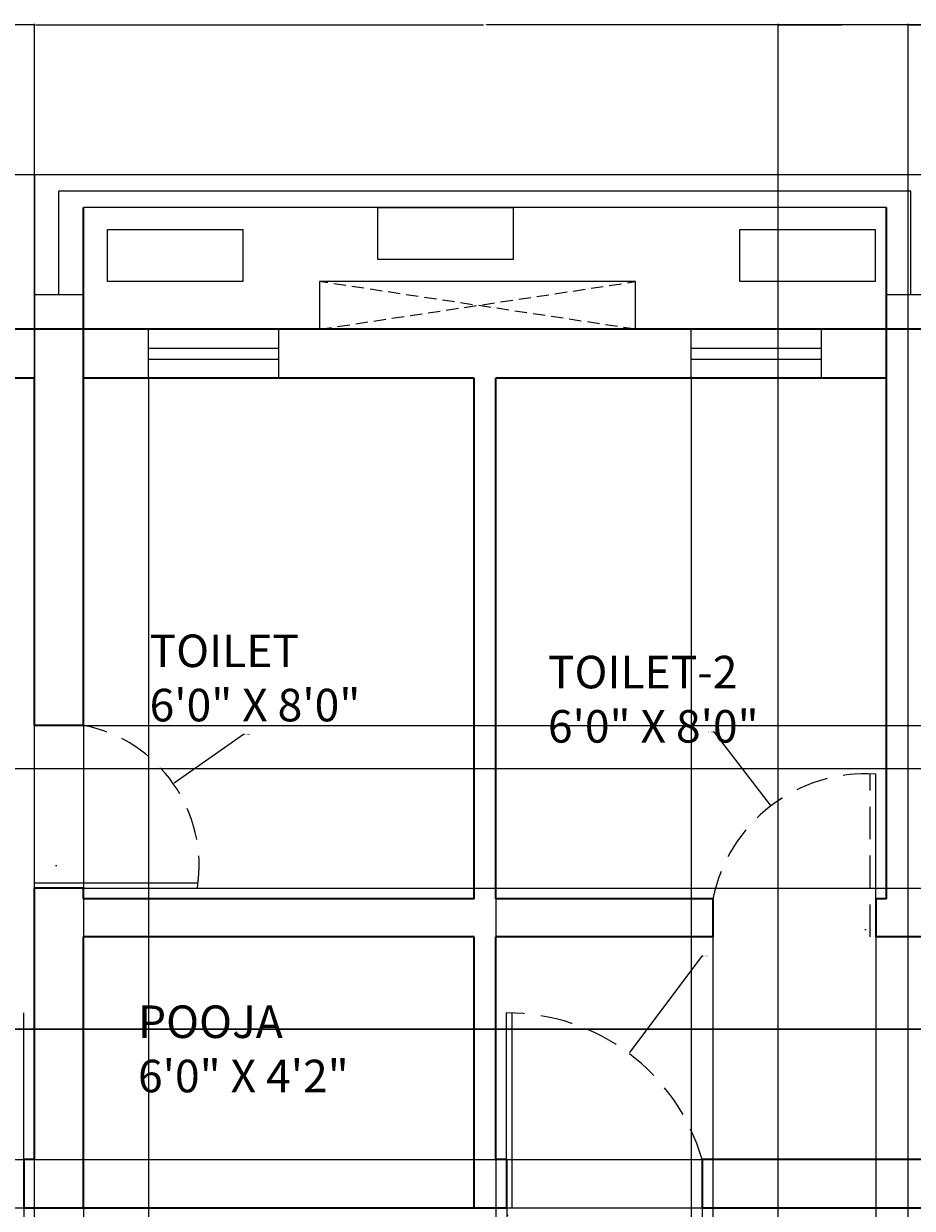
# Model space of a CAD drawing. Units: inches. Extents: x 6662 to 7211, y 5077 to 5683.
# Tile 8 of 9: x 6868 to 7032, y 5465 to 5683. Entities that reach past the tile are written whole.
import ezdxf

# ---------------------------------------------------------------- set-up
doc = ezdxf.new("R2010")
doc.units = ezdxf.units.IN
doc.header["$LTSCALE"] = 3
doc.header["$MEASUREMENT"] = 0
doc.linetypes.add('HIDDEN', pattern=[0.375, 0.25, -0.125])
for name, color, linetype, lineweight in [('A-ANNO-DIMS', 2, 'Continuous', 18), ('A-AREA-IDEN', 7, 'Continuous', 18), ('A-DOOR', 4, 'Continuous', 25), ('A-DOOR-HIDN', 4, 'HIDDEN', 13), ('A-FLOR-CASE-PATT', 241, 'Continuous', 13), ('A-FLOR-PROJ', 7, 'Continuous', 18), ('A-FLOR-PROJ-HIDN', 7, 'HIDDEN', 13), ('A-GLAZ', 4, 'Continuous', 18), ('A-WALL', 7, 'Continuous', 35)]:
    doc.layers.add(name, color=color, linetype=linetype, lineweight=lineweight)
doc.styles.get("Standard").update_dxf_attribs({"font": 'arial.ttf'})
doc.dimstyles.get("Standard").update_dxf_attribs({"dimtxt": 0.18, "dimasz": 0.18, "dimexe": 0.18, "dimexo": 0.0625, "dimgap": 0.09, "dimtad": 0, "dimtih": 1, "dimtoh": 1, "dimdec": 4, "dimzin": 0, "dimdsep": 46, "dimtxsty": 'Standard', "dimcen": 0.09, "dimadec": 0, "dimazin": 0, "dimtfac": 1, "dimtdec": 4, "dimtofl": 0, "dimtmove": 0, "dimatfit": 3, "dimfxl": 1, "dimtolj": 1, "dimtzin": 0, "dimarcsym": 0})

# ---------------------------------------------------------------- blocks, each defined once
blk = doc.blocks.new('WIN-VENT-24IN')
for p, q in [((0, 0), (0, 9)), ((24, 0), (24, 9)), ((0, 5.5), (24, 5.5)), ((0, 3.5), (24, 3.5))]:
    blk.add_line(p, q)
blk = doc.blocks.new('*D41')
at = {"layer": 'A-ANNO-DIMS', "color": 0, "lineweight": -2, "ltscale": 3, "transparency": 16777216}
for p, q in [((7035.92, 5655.02), (7210.74, 5655.02)), ((7210.56, 5654.84), (7210.56, 5379.99)), ((7210.56, 5104.78), (7210.56, 5379.63)), ((7010.92, 5104.6), (7210.74, 5104.6))]:
    blk.add_line(p, q, dxfattribs=at)
at = {"layer": 'A-ANNO-DIMS', "color": 0, "ltscale": 3, "transparency": 16777216}
for points in [[(7210.53, 5654.84), (7210.59, 5654.84), (7210.56, 5655.02)], [(7210.53, 5104.78), (7210.59, 5104.78), (7210.56, 5104.6)]]:
    blk.add_solid(points, dxfattribs=at)
at = {"layer": 'Defpoints', "color": 0, "ltscale": 3, "transparency": 16777216}
for p in [(7035.86, 5655.02), (7210.56, 5655.02), (7010.86, 5104.6)]:
    blk.add_point(p, dxfattribs=at)
at = {"layer": 'A-ANNO-DIMS', "color": 0, "ltscale": 3, "transparency": 16777216, "insert": (7210.56, 5379.81), "char_height": 0.18, "attachment_point": 5}
blk.add_mtext('\\A1;550.4', dxfattribs=at)
blk = doc.blocks.new('*D45')
at = {"layer": 'A-ANNO-DIMS', "color": 0, "lineweight": -2, "ltscale": 3, "transparency": 16777216}
for p, q in [((6845.86, 5626.66), (6845.86, 5682.9)), ((6846.04, 5682.72), (6857.64, 5682.72)), ((6869.68, 5682.72), (6858.08, 5682.72)), ((6869.86, 5655.08), (6869.86, 5682.9))]:
    blk.add_line(p, q, dxfattribs=at)
at = {"layer": 'A-ANNO-DIMS', "color": 0, "ltscale": 3, "transparency": 16777216}
for points in [[(6846.04, 5682.75), (6846.04, 5682.69), (6845.86, 5682.72)], [(6869.68, 5682.75), (6869.68, 5682.69), (6869.86, 5682.72)]]:
    blk.add_solid(points, dxfattribs=at)
at = {"layer": 'Defpoints', "color": 0, "ltscale": 3, "transparency": 16777216}
for p in [(6869.86, 5682.72), (6869.86, 5655.02), (6845.86, 5626.6)]:
    blk.add_point(p, dxfattribs=at)
at = {"layer": 'A-ANNO-DIMS', "color": 0, "ltscale": 3, "transparency": 16777216, "insert": (6857.86, 5682.72), "char_height": 0.18, "attachment_point": 5}
blk.add_mtext('\\A1;24', dxfattribs=at)
blk = doc.blocks.new('*D46')
at = {"layer": 'A-ANNO-DIMS', "color": 0, "lineweight": -2, "ltscale": 3, "transparency": 16777216}
for p, q in [((6869.86, 5655.08), (6869.86, 5682.9)), ((6870.04, 5682.72), (6952.58, 5682.72)), ((7035.68, 5682.72), (6953.14, 5682.72)), ((7035.86, 5655.08), (7035.86, 5682.9))]:
    blk.add_line(p, q, dxfattribs=at)
at = {"layer": 'A-ANNO-DIMS', "color": 0, "ltscale": 3, "transparency": 16777216}
for points in [[(6870.04, 5682.75), (6870.04, 5682.69), (6869.86, 5682.72)], [(7035.68, 5682.75), (7035.68, 5682.69), (7035.86, 5682.72)]]:
    blk.add_solid(points, dxfattribs=at)
at = {"layer": 'Defpoints', "color": 0, "ltscale": 3, "transparency": 16777216}
for p in [(7035.86, 5682.72), (6869.86, 5655.02), (7035.86, 5655.02)]:
    blk.add_point(p, dxfattribs=at)
at = {"layer": 'A-ANNO-DIMS', "color": 0, "ltscale": 3, "transparency": 16777216, "insert": (6952.86, 5682.72), "char_height": 0.18, "attachment_point": 5}
blk.add_mtext('\\A1;166', dxfattribs=at)
blk = doc.blocks.new('*D50')
at = {"layer": 'A-ANNO-DIMS', "color": 0, "lineweight": -2, "ltscale": 3, "transparency": 16777216}
for p, q in [((6869.8, 5655.02), (6661.98, 5655.02)), ((6662.16, 5654.84), (6662.16, 5640.99)), ((6662.16, 5626.78), (6662.16, 5640.63)), ((6716.8, 5626.6), (6661.98, 5626.6))]:
    blk.add_line(p, q, dxfattribs=at)
at = {"layer": 'A-ANNO-DIMS', "color": 0, "ltscale": 3, "transparency": 16777216}
for points in [[(6662.13, 5654.84), (6662.19, 5654.84), (6662.16, 5655.02)], [(6662.13, 5626.78), (6662.19, 5626.78), (6662.16, 5626.6)]]:
    blk.add_solid(points, dxfattribs=at)
at = {"layer": 'Defpoints', "color": 0, "ltscale": 3, "transparency": 16777216}
for p in [(6662.16, 5655.02), (6869.86, 5655.02), (6716.86, 5626.6)]:
    blk.add_point(p, dxfattribs=at)
at = {"layer": 'A-ANNO-DIMS', "color": 0, "ltscale": 3, "transparency": 16777216, "insert": (6662.16, 5640.81), "char_height": 0.18, "attachment_point": 5}
blk.add_mtext('\\A1;28.423', dxfattribs=at)
blk = doc.blocks.new('*D64')
at = {"layer": 'A-ANNO-DIMS', "color": 0, "lineweight": -2, "ltscale": 3, "transparency": 16777216}
for p, q in [((6833.86, 5332.16), (6833.86, 5682.9)), ((6834.04, 5682.72), (6851.64, 5682.72)), ((6869.68, 5682.72), (6852.08, 5682.72)), ((6869.86, 5332.16), (6869.86, 5682.9))]:
    blk.add_line(p, q, dxfattribs=at)
at = {"layer": 'A-ANNO-DIMS', "color": 0, "ltscale": 3, "transparency": 16777216}
for points in [[(6834.04, 5682.75), (6834.04, 5682.69), (6833.86, 5682.72)], [(6869.68, 5682.75), (6869.68, 5682.69), (6869.86, 5682.72)]]:
    blk.add_solid(points, dxfattribs=at)
at = {"layer": 'Defpoints', "color": 0, "ltscale": 3, "transparency": 16777216}
for p in [(6869.86, 5682.72), (6833.86, 5332.1), (6869.86, 5332.1)]:
    blk.add_point(p, dxfattribs=at)
at = {"layer": 'A-ANNO-DIMS', "color": 0, "ltscale": 3, "transparency": 16777216, "insert": (6851.86, 5682.72), "char_height": 0.18, "attachment_point": 5}
blk.add_mtext('\\A1;36', dxfattribs=at)
blk = doc.blocks.new('*D65')
at = {"layer": 'A-ANNO-DIMS', "color": 0, "lineweight": -2, "ltscale": 3, "transparency": 16777216}
for p, q in [((6831.86, 5464.54), (6831.86, 5076.72)), ((6867.86, 5464.54), (6867.86, 5076.72)), ((6832.04, 5076.9), (6849.64, 5076.9)), ((6867.68, 5076.9), (6850.08, 5076.9))]:
    blk.add_line(p, q, dxfattribs=at)
at = {"layer": 'A-ANNO-DIMS', "color": 0, "ltscale": 3, "transparency": 16777216}
for points in [[(6832.04, 5076.93), (6832.04, 5076.87), (6831.86, 5076.9)], [(6867.68, 5076.93), (6867.68, 5076.87), (6867.86, 5076.9)]]:
    blk.add_solid(points, dxfattribs=at)
at = {"layer": 'Defpoints', "color": 0, "ltscale": 3, "transparency": 16777216}
for p in [(6831.86, 5464.6), (6867.86, 5464.6), (6867.86, 5076.9)]:
    blk.add_point(p, dxfattribs=at)
at = {"layer": 'A-ANNO-DIMS', "color": 0, "ltscale": 3, "transparency": 16777216, "insert": (6849.86, 5076.9), "char_height": 0.18, "attachment_point": 5}
blk.add_mtext('\\A1;36', dxfattribs=at)
blk = doc.blocks.new('*D66')
at = {"layer": 'A-ANNO-DIMS', "color": 0, "lineweight": -2, "ltscale": 3, "transparency": 16777216}
for p, q in [((6956.86, 5464.54), (6956.86, 5076.72)), ((6992.86, 5464.54), (6992.86, 5076.72)), ((6957.04, 5076.9), (6974.64, 5076.9)), ((6992.68, 5076.9), (6975.08, 5076.9))]:
    blk.add_line(p, q, dxfattribs=at)
at = {"layer": 'A-ANNO-DIMS', "color": 0, "ltscale": 3, "transparency": 16777216}
for points in [[(6957.04, 5076.93), (6957.04, 5076.87), (6956.86, 5076.9)], [(6992.68, 5076.93), (6992.68, 5076.87), (6992.86, 5076.9)]]:
    blk.add_solid(points, dxfattribs=at)
at = {"layer": 'Defpoints', "color": 0, "ltscale": 3, "transparency": 16777216}
for p in [(6956.86, 5464.6), (6992.86, 5464.6), (6992.86, 5076.9)]:
    blk.add_point(p, dxfattribs=at)
at = {"layer": 'A-ANNO-DIMS', "color": 0, "ltscale": 3, "transparency": 16777216, "insert": (6974.86, 5076.9), "char_height": 0.18, "attachment_point": 5}
blk.add_mtext('\\A1;36', dxfattribs=at)
blk = doc.blocks.new('*D67')
at = {"layer": 'A-ANNO-DIMS', "color": 0, "lineweight": -2, "ltscale": 3, "transparency": 16777216}
for p, q in [((6994.86, 5514.54), (6994.86, 5076.72)), ((7024.86, 5514.54), (7024.86, 5076.72)), ((6995.04, 5076.9), (7009.64, 5076.9)), ((7024.68, 5076.9), (7010.08, 5076.9))]:
    blk.add_line(p, q, dxfattribs=at)
at = {"layer": 'A-ANNO-DIMS', "color": 0, "ltscale": 3, "transparency": 16777216}
for points in [[(6995.04, 5076.93), (6995.04, 5076.87), (6994.86, 5076.9)], [(7024.68, 5076.93), (7024.68, 5076.87), (7024.86, 5076.9)]]:
    blk.add_solid(points, dxfattribs=at)
at = {"layer": 'Defpoints', "color": 0, "ltscale": 3, "transparency": 16777216}
for p in [(6994.86, 5514.6), (7024.86, 5514.6), (7024.86, 5076.9)]:
    blk.add_point(p, dxfattribs=at)
at = {"layer": 'A-ANNO-DIMS', "color": 0, "ltscale": 3, "transparency": 16777216, "insert": (7009.86, 5076.9), "char_height": 0.18, "attachment_point": 5}
blk.add_mtext('\\A1;30', dxfattribs=at)
blk = doc.blocks.new('*D68')
at = {"layer": 'A-ANNO-DIMS', "color": 0, "lineweight": -2, "ltscale": 3, "transparency": 16777216}
for p, q in [((6878.92, 5553.6), (7210.74, 5553.6)), ((7210.56, 5553.42), (7210.56, 5538.78)), ((7210.56, 5523.78), (7210.56, 5538.42)), ((6878.92, 5523.6), (7210.74, 5523.6))]:
    blk.add_line(p, q, dxfattribs=at)
at = {"layer": 'A-ANNO-DIMS', "color": 0, "ltscale": 3, "transparency": 16777216}
for points in [[(7210.53, 5553.42), (7210.59, 5553.42), (7210.56, 5553.6)], [(7210.53, 5523.78), (7210.59, 5523.78), (7210.56, 5523.6)]]:
    blk.add_solid(points, dxfattribs=at)
at = {"layer": 'Defpoints', "color": 0, "ltscale": 3, "transparency": 16777216}
for p in [(6878.86, 5553.6), (7210.56, 5553.6), (6878.86, 5523.6)]:
    blk.add_point(p, dxfattribs=at)
at = {"layer": 'A-ANNO-DIMS', "color": 0, "ltscale": 3, "transparency": 16777216, "insert": (7210.56, 5538.6), "char_height": 0.18, "attachment_point": 5}
blk.add_mtext('\\A1;30', dxfattribs=at)
blk = doc.blocks.new('*D71')
at = {"layer": 'A-ANNO-DIMS', "color": 0, "lineweight": -2, "ltscale": 3, "transparency": 16777216}
for p, q in [((6878.86, 5617.54), (6878.86, 5076.72)), ((6890.86, 5617.54), (6890.86, 5076.72)), ((6879.04, 5076.9), (6884.65, 5076.9)), ((6890.68, 5076.9), (6885.07, 5076.9))]:
    blk.add_line(p, q, dxfattribs=at)
at = {"layer": 'A-ANNO-DIMS', "color": 0, "ltscale": 3, "transparency": 16777216}
for points in [[(6879.04, 5076.93), (6879.04, 5076.87), (6878.86, 5076.9)], [(6890.68, 5076.93), (6890.68, 5076.87), (6890.86, 5076.9)]]:
    blk.add_solid(points, dxfattribs=at)
at = {"layer": 'Defpoints', "color": 0, "ltscale": 3, "transparency": 16777216}
for p in [(6878.86, 5617.6), (6890.86, 5617.6), (6878.86, 5076.9)]:
    blk.add_point(p, dxfattribs=at)
at = {"layer": 'A-ANNO-DIMS', "color": 0, "ltscale": 3, "transparency": 16777216, "insert": (6884.86, 5076.9), "char_height": 0.18, "attachment_point": 5}
blk.add_mtext('\\A1;12', dxfattribs=at)
blk = doc.blocks.new('*D72')
at = {"layer": 'A-ANNO-DIMS', "color": 0, "lineweight": -2, "ltscale": 3, "transparency": 16777216}
for p, q in [((6954.86, 5617.54), (6954.86, 5076.72)), ((6990.86, 5617.54), (6990.86, 5076.72)), ((6955.04, 5076.9), (6972.64, 5076.9)), ((6990.68, 5076.9), (6973.08, 5076.9))]:
    blk.add_line(p, q, dxfattribs=at)
at = {"layer": 'A-ANNO-DIMS', "color": 0, "ltscale": 3, "transparency": 16777216}
for points in [[(6955.04, 5076.93), (6955.04, 5076.87), (6954.86, 5076.9)], [(6990.68, 5076.93), (6990.68, 5076.87), (6990.86, 5076.9)]]:
    blk.add_solid(points, dxfattribs=at)
at = {"layer": 'Defpoints', "color": 0, "ltscale": 3, "transparency": 16777216}
for p in [(6954.86, 5617.6), (6990.86, 5617.6), (6990.86, 5076.9)]:
    blk.add_point(p, dxfattribs=at)
at = {"layer": 'A-ANNO-DIMS', "color": 0, "ltscale": 3, "transparency": 16777216, "insert": (6972.86, 5076.9), "char_height": 0.18, "attachment_point": 5}
blk.add_mtext('\\A1;36', dxfattribs=at)
blk = doc.blocks.new('*D74')
at = {"layer": 'A-ANNO-DIMS', "color": 0, "lineweight": -2, "ltscale": 3, "transparency": 16777216}
for p, q in [((7006.86, 5179.16), (7006.86, 5682.9)), ((7007.04, 5682.72), (7018.64, 5682.72)), ((7030.68, 5682.72), (7019.08, 5682.72)), ((7030.86, 5179.16), (7030.86, 5682.9))]:
    blk.add_line(p, q, dxfattribs=at)
at = {"layer": 'A-ANNO-DIMS', "color": 0, "ltscale": 3, "transparency": 16777216}
for points in [[(7007.04, 5682.75), (7007.04, 5682.69), (7006.86, 5682.72)], [(7030.68, 5682.75), (7030.68, 5682.69), (7030.86, 5682.72)]]:
    blk.add_solid(points, dxfattribs=at)
at = {"layer": 'Defpoints', "color": 0, "ltscale": 3, "transparency": 16777216}
for p in [(7030.86, 5682.72), (7006.86, 5179.1), (7030.86, 5179.1)]:
    blk.add_point(p, dxfattribs=at)
at = {"layer": 'A-ANNO-DIMS', "color": 0, "ltscale": 3, "transparency": 16777216, "insert": (7018.86, 5682.72), "char_height": 0.18, "attachment_point": 5}
blk.add_mtext('\\A1;24', dxfattribs=at)
blk = doc.blocks.new('*D75')
at = {"layer": 'A-ANNO-DIMS', "color": 0, "lineweight": -2, "ltscale": 3, "transparency": 16777216}
for p, q in [((7030.86, 5179.16), (7030.86, 5682.9)), ((7031.04, 5682.72), (7054.64, 5682.72)), ((7078.68, 5682.72), (7055.08, 5682.72)), ((7078.86, 5179.16), (7078.86, 5682.9))]:
    blk.add_line(p, q, dxfattribs=at)
at = {"layer": 'A-ANNO-DIMS', "color": 0, "ltscale": 3, "transparency": 16777216}
for points in [[(7031.04, 5682.75), (7031.04, 5682.69), (7030.86, 5682.72)], [(7078.68, 5682.75), (7078.68, 5682.69), (7078.86, 5682.72)]]:
    blk.add_solid(points, dxfattribs=at)
at = {"layer": 'Defpoints', "color": 0, "ltscale": 3, "transparency": 16777216}
for p in [(7078.86, 5682.72), (7030.86, 5179.1), (7078.86, 5179.1)]:
    blk.add_point(p, dxfattribs=at)
at = {"layer": 'A-ANNO-DIMS', "color": 0, "ltscale": 3, "transparency": 16777216, "insert": (7054.86, 5682.72), "char_height": 0.18, "attachment_point": 5}
blk.add_mtext('\\A1;48', dxfattribs=at)
blk = doc.blocks.new('*D76')
at = {"layer": 'A-ANNO-DIMS', "color": 0, "lineweight": -2, "ltscale": 3, "transparency": 16777216}
for p, q in [((7167.8, 5464.6), (6661.98, 5464.6)), ((6662.16, 5464.42), (6662.16, 5449.65)), ((6662.16, 5434.53), (6662.16, 5449.29)), ((7167.8, 5434.35), (6661.98, 5434.35))]:
    blk.add_line(p, q, dxfattribs=at)
at = {"layer": 'A-ANNO-DIMS', "color": 0, "ltscale": 3, "transparency": 16777216}
for points in [[(6662.13, 5464.42), (6662.19, 5464.42), (6662.16, 5464.6)], [(6662.13, 5434.53), (6662.19, 5434.53), (6662.16, 5434.35)]]:
    blk.add_solid(points, dxfattribs=at)
at = {"layer": 'Defpoints', "color": 0, "ltscale": 3, "transparency": 16777216}
for p in [(7167.86, 5464.6), (6662.16, 5434.35), (7167.86, 5434.35)]:
    blk.add_point(p, dxfattribs=at)
at = {"layer": 'A-ANNO-DIMS', "color": 0, "ltscale": 3, "transparency": 16777216, "insert": (6662.16, 5449.47), "char_height": 0.18, "attachment_point": 5}
blk.add_mtext('\\A1;30.25', dxfattribs=at)
blk = doc.blocks.new('*D80')
at = {"layer": 'A-ANNO-DIMS', "color": 0, "lineweight": -2, "ltscale": 3, "transparency": 16777216}
for p, q in [((6825.96, 5497.6), (7210.74, 5497.6)), ((7210.56, 5497.42), (7210.56, 5485.78)), ((7210.56, 5473.78), (7210.56, 5485.42)), ((6825.96, 5473.6), (7210.74, 5473.6))]:
    blk.add_line(p, q, dxfattribs=at)
at = {"layer": 'A-ANNO-DIMS', "color": 0, "ltscale": 3, "transparency": 16777216}
for points in [[(7210.53, 5497.42), (7210.59, 5497.42), (7210.56, 5497.6)], [(7210.53, 5473.78), (7210.59, 5473.78), (7210.56, 5473.6)]]:
    blk.add_solid(points, dxfattribs=at)
at = {"layer": 'Defpoints', "color": 0, "ltscale": 3, "transparency": 16777216}
for p in [(6825.9, 5497.6), (7210.56, 5497.6), (6825.9, 5473.6)]:
    blk.add_point(p, dxfattribs=at)
at = {"layer": 'A-ANNO-DIMS', "color": 0, "ltscale": 3, "transparency": 16777216, "insert": (7210.56, 5485.6), "char_height": 0.18, "attachment_point": 5}
blk.add_mtext('\\A1;24', dxfattribs=at)
blk = doc.blocks.new('*D82')
at = {"layer": 'A-ANNO-DIMS', "color": 0, "lineweight": -2, "ltscale": 3, "transparency": 16777216}
for p, q in [((7167.8, 5545.6), (6661.98, 5545.6)), ((6662.16, 5545.42), (6662.16, 5521.78)), ((6662.16, 5497.78), (6662.16, 5521.42)), ((7167.8, 5497.6), (6661.98, 5497.6))]:
    blk.add_line(p, q, dxfattribs=at)
at = {"layer": 'A-ANNO-DIMS', "color": 0, "ltscale": 3, "transparency": 16777216}
for points in [[(6662.13, 5545.42), (6662.19, 5545.42), (6662.16, 5545.6)], [(6662.13, 5497.78), (6662.19, 5497.78), (6662.16, 5497.6)]]:
    blk.add_solid(points, dxfattribs=at)
at = {"layer": 'Defpoints', "color": 0, "ltscale": 3, "transparency": 16777216}
for p in [(6662.16, 5545.6), (7167.86, 5545.6), (7167.86, 5497.6)]:
    blk.add_point(p, dxfattribs=at)
at = {"layer": 'A-ANNO-DIMS', "color": 0, "ltscale": 3, "transparency": 16777216, "insert": (6662.16, 5521.6), "char_height": 0.18, "attachment_point": 5}
blk.add_mtext('\\A1;48', dxfattribs=at)
blk = doc.blocks.new('*D88')
at = {"layer": 'A-ANNO-DIMS', "color": 0, "lineweight": -2, "ltscale": 3, "transparency": 16777216}
for p, q in [((6992.81, 5511.04), (6979.5, 5493.29)), ((6992.99, 5511.04), (6992.81, 5511.04)), ((6956.93, 5463.31), (6957.11, 5463.31)), ((6957.02, 5463.22), (6957.02, 5463.4))]:
    blk.add_line(p, q, dxfattribs=at)
at = {"layer": 'A-ANNO-DIMS', "color": 0, "ltscale": 3, "transparency": 16777216}
blk.add_solid([(6979.47, 5493.3), (6979.52, 5493.27), (6979.39, 5493.14)], dxfattribs=at)
at = {"layer": 'Defpoints', "color": 0, "ltscale": 3, "transparency": 16777216}
for p in [(6979.39, 5493.14), (6957.02, 5463.31)]:
    blk.add_point(p, dxfattribs=at)
at = {"layer": 'A-ANNO-DIMS', "color": 0, "ltscale": 3, "transparency": 16777216, "insert": (6993.54, 5511.04), "char_height": 0.18, "attachment_point": 5}
blk.add_mtext('\\A1;R37.285', dxfattribs=at)
blk = doc.blocks.new('*D93')
at = {"layer": 'A-ANNO-DIMS', "color": 0, "lineweight": -2, "ltscale": 3, "transparency": 16777216}
for p, q in [((6994.88, 5552.4), (6995.06, 5552.4)), ((6995.06, 5552.4), (7005.42, 5538.88)), ((7022.9, 5515.97), (7023.08, 5515.97)), ((7022.99, 5515.88), (7022.99, 5516.06))]:
    blk.add_line(p, q, dxfattribs=at)
at = {"layer": 'A-ANNO-DIMS', "color": 0, "ltscale": 3, "transparency": 16777216}
blk.add_solid([(7005.45, 5538.9), (7005.4, 5538.86), (7005.53, 5538.74)], dxfattribs=at)
at = {"layer": 'Defpoints', "color": 0, "ltscale": 3, "transparency": 16777216}
for p in [(7005.53, 5538.74), (7022.99, 5515.97)]:
    blk.add_point(p, dxfattribs=at)
at = {"layer": 'A-ANNO-DIMS', "color": 0, "ltscale": 3, "transparency": 16777216, "insert": (6994.4, 5552.4), "char_height": 0.18, "attachment_point": 5}
blk.add_mtext('\\A1;R28.69', dxfattribs=at)
blk = doc.blocks.new('*D95')
at = {"layer": 'A-ANNO-DIMS', "color": 0, "lineweight": -2, "ltscale": 3, "transparency": 16777216}
for p, q in [((6908.37, 5551.9), (6895.58, 5542.95)), ((6908.55, 5551.9), (6908.37, 5551.9)), ((6873.78, 5527.76), (6873.96, 5527.76)), ((6873.87, 5527.67), (6873.87, 5527.85))]:
    blk.add_line(p, q, dxfattribs=at)
at = {"layer": 'A-ANNO-DIMS', "color": 0, "ltscale": 3, "transparency": 16777216}
blk.add_solid([(6895.56, 5542.98), (6895.6, 5542.93), (6895.43, 5542.85)], dxfattribs=at)
at = {"layer": 'Defpoints', "color": 0, "ltscale": 3, "transparency": 16777216}
for p in [(6895.43, 5542.85), (6873.87, 5527.76)]:
    blk.add_point(p, dxfattribs=at)
at = {"layer": 'A-ANNO-DIMS', "color": 0, "ltscale": 3, "transparency": 16777216, "insert": (6909.1, 5551.9), "char_height": 0.18, "attachment_point": 5}
blk.add_mtext('\\A1;R26.315', dxfattribs=at)

msp = doc.modelspace()

# ---------------------------------------------------------------- hatches: boundary and pattern name
at = {"layer": 'A-FLOR-CASE-PATT'}
h = msp.add_hatch(dxfattribs=at)
h.set_pattern_fill('ANSI31', color=256)
h.paths.add_polyline_path([(6869.8579, 5283.7981), (6845.8579, 5283.7981), (6845.8579, 5229.4653), (6847.018, 5229.7817, -0.54116316), (6849.0925, 5228.1371), (6849.7129, 5228.234, -0.50821327), (6851.018, 5227.2817), (6851.018, 5226.7817), (6855.018, 5227.2817), (6855.018, 5225.7817), (6851.018, 5225.2817), (6851.018, 5217.7817), (6851.018, 5210.2817), (6855.018, 5209.7817), (6855.018, 5208.2817), (6851.018, 5208.7817), (6851.018, 5208.2817, -0.41421356), (6850.018, 5207.2817), (6849.0925, 5207.4263, -0.50580924), (6847.1872, 5205.7355), (6845.8579, 5206.0981), (6845.8579, 5179.0979), (6869.8579, 5179.0979)])
h.paths.add_polyline_path([(7167.8579, 5497.5979), (7143.8579, 5497.5979), (7078.3579, 5497.5979), (7078.3579, 5473.5979), (7163.8579, 5473.5979), (7167.8579, 5473.5979)])
h.paths.add_polyline_path([(6825.9016, 5497.5979), (6725.8579, 5497.5979), (6725.8579, 5473.5979), (6825.9016, 5473.5979)])
h.paths.add_polyline_path([(6796.6359, 5485.2095), (6797.1359, 5489.2095), (6806.1359, 5489.2095), (6815.1359, 5489.2095), (6815.6359, 5485.2095), (6814.1359, 5485.2095), (6813.6359, 5489.2095), (6806.1359, 5489.2095), (6798.6359, 5489.2095), (6798.1359, 5485.2095)], flags=16)

# ---------------------------------------------------------------- linework, layer by layer
at = {"layer": 'A-DOOR'}
for p, q in [((7024.8579, 5514.5979), (7024.8579, 5544.5979)), ((6869.8579, 5524.5979), (6899.8579, 5524.5979)), ((6869.8579, 5523.5979), (6899.8579, 5523.5979)), ((6867.8579, 5464.5979), (6867.8579, 5500.5979)), ((6956.8579, 5464.5979), (6956.8579, 5500.5979)), ((6957.8579, 5464.5979), (6957.8579, 5500.5979))]:
    msp.add_line(p, q, dxfattribs=at)
at = {"layer": 'A-DOOR-HIDN', "ltscale": 8}
msp.add_line((7023.8579, 5514.5979), (7023.8579, 5544.5979), dxfattribs=at)
for centre, radius, start, end in [((6873.8742, 5527.7594), 26.3148, 350.900982, 79.083059), ((7022.9889, 5515.9706), 28.6883, 86.264613, 168.687746), ((6957.0195, 5463.3135), 37.2848, 16.011746, 90.248459)]:
    msp.add_arc(centre, radius, start, end, dxfattribs=at)
at = {"layer": 'A-FLOR-PROJ', "ltscale": 3}
for p, q in [((6869.8579, 5655.0209), (6869.8579, 5617.5979)), ((6950.8579, 5655.0209), (6869.8579, 5655.0209)), ((7035.8579, 5655.0209), (6950.8579, 5655.0209)), ((6950.8579, 5652.0209), (6874.3579, 5652.0209)), ((6874.3579, 5633.0136), (6874.3579, 5652.0209)), ((7031.3579, 5652.0209), (6950.8579, 5652.0209)), ((7031.3579, 5633.0136), (7031.3579, 5652.0209)), ((6950.8579, 5649.0209), (6878.8579, 5649.0209)), ((7026.8579, 5649.0209), (6950.8579, 5649.0209)), ((6869.8579, 5633.0136), (6878.8579, 5633.0136)), ((7026.8579, 5633.0136), (7035.8579, 5633.0136))]:
    msp.add_line(p, q, dxfattribs=at)
for points in [[(6933.0868, 5649.0209), (6958.0554, 5649.0209), (6958.0554, 5639.4448), (6933.0868, 5639.4448)], [(6883.2757, 5644.9491), (6908.2443, 5644.9491), (6908.2443, 5635.373), (6883.2757, 5635.373)], [(6999.7959, 5644.9491), (7024.7645, 5644.9491), (7024.7645, 5635.373), (6999.7959, 5635.373)], [(6922.368, 5626.5979), (6980.6281, 5626.5979), (6980.6281, 5635.373), (6922.368, 5635.373)]]:
    msp.add_lwpolyline(points, close=True, dxfattribs=at)
at = {"layer": 'A-FLOR-PROJ-HIDN', "ltscale": 3}
for p, q in [((6922.368, 5626.5979), (6980.6281, 5635.373)), ((6980.6281, 5626.5979), (6922.368, 5635.373))]:
    msp.add_line(p, q, dxfattribs=at)
at = {"layer": 'A-WALL'}
for p, q in [((6878.8579, 5553.5979), (6878.8579, 5649.0209)), ((7026.8579, 5521.5979), (7026.8579, 5649.0209)), ((7176.8579, 5626.5979), (6716.8579, 5626.5979)), ((6869.8579, 5617.5979), (6725.8579, 5617.5979)), ((6869.8579, 5553.5979), (6869.8579, 5617.5979)), ((6950.8579, 5617.5979), (6878.8579, 5617.5979)), ((6950.8579, 5521.5979), (6950.8579, 5617.5979)), ((7026.8579, 5617.5979), (6954.8579, 5617.5979)), ((6954.8579, 5521.5979), (6954.8579, 5617.5979)), ((6878.8579, 5553.5979), (6869.8579, 5553.5979)), ((6869.8579, 5473.5979), (6869.8579, 5523.5979)), ((6878.8579, 5523.5979), (6869.8579, 5523.5979)), ((6878.8579, 5521.5979), (6878.8579, 5523.5979)), ((6950.8579, 5521.5979), (6878.8579, 5521.5979)), ((6994.8579, 5521.5979), (6954.8579, 5521.5979)), ((6994.8579, 5521.5979), (6994.8579, 5514.5979)), ((7026.8579, 5521.5979), (7024.8579, 5521.5979)), ((7024.8579, 5521.5979), (7024.8579, 5514.5979)), ((6878.8579, 5464.5979), (6878.8579, 5514.5979)), ((6950.8579, 5514.5979), (6878.8579, 5514.5979)), ((6950.8579, 5464.5979), (6950.8579, 5514.5979)), ((6954.8579, 5473.5979), (6954.8579, 5514.5979)), ((6994.8579, 5514.5979), (6954.8579, 5514.5979)), ((7035.8579, 5514.5979), (7024.8579, 5514.5979)), ((6869.8579, 5473.5979), (6867.8579, 5473.5979)), ((6867.8579, 5473.5979), (6867.8579, 5464.5979)), ((6956.8579, 5473.5979), (6954.8579, 5473.5979)), ((6956.8579, 5473.5979), (6956.8579, 5464.5979)), ((7163.8579, 5473.5979), (6992.8579, 5473.5979)), ((6992.8579, 5473.5979), (6992.8579, 5464.5979)), ((6956.8579, 5464.5979), (6867.8579, 5464.5979)), ((6956.8579, 5464.5979), (6867.8579, 5464.5979)), ((6869.8579, 5464.5979), (6869.8579, 5464.5979)), ((7106.8579, 5464.5979), (6992.8579, 5464.5979))]:
    msp.add_line(p, q, dxfattribs=at)

# ---------------------------------------------------------------- block references
at = {"layer": 'A-GLAZ'}
for p in [(6890.858, 5617.598), (6990.858, 5617.598)]:
    msp.add_blockref('WIN-VENT-24IN', p, dxfattribs=at)

# ---------------------------------------------------------------- texts
at = {"layer": 'A-AREA-IDEN', "ltscale": 3, "char_height": 6, "attachment_point": 1}
for s, insert in [('TOILET\\P6\'0" X 8\'0"', (6891.0556, 5570.3336)), ('TOILET-2\\P6\'0" X 8\'0"', (6964.4536, 5566.4175)), ('POOJA\\P6\'0" X 4\'2"', (6888.9178, 5501.9798))]:
    msp.add_mtext_dynamic_manual_height_columns(s, width=381.547883, gutter_width=1, heights=[0], dxfattribs=dict(at, insert=insert))

# ---------------------------------------------------------------- dimensions: what is measured, and where the dimension line sits
at = {"layer": 'A-ANNO-DIMS', "ltscale": 3}
for base, p1, p2, picture, middle in [((6869.8579, 5682.7209), (6833.8579, 5332.0979), (6869.8579, 5332.0979), '*D64', (6851.8579, 5682.7209)), ((6869.8579, 5682.7209), (6845.8579, 5626.5979), (6869.8579, 5655.0209), '*D45', (6857.8579, 5682.7209)), ((7035.8579, 5682.7209), (6869.8579, 5655.0209), (7035.8579, 5655.0209), '*D46', (6952.8579, 5682.7209)), ((7030.8579, 5682.7209), (7006.8579, 5179.0979), (7030.8579, 5179.0979), '*D74', (7018.8579, 5682.7209)), ((7078.8579, 5682.7209), (7030.8579, 5179.0979), (7078.8579, 5179.0979), '*D75', (7054.8579, 5682.7209)), ((6878.8579, 5076.8979), (6890.8579, 5617.5979), (6878.8579, 5617.5979), '*D71', (6884.8579, 5076.8979)), ((6990.8579, 5076.8979), (6954.8579, 5617.5979), (6990.8579, 5617.5979), '*D72', (6972.8579, 5076.8979)), ((7024.8579, 5076.8979), (6994.8579, 5514.5979), (7024.8579, 5514.5979), '*D67', (7009.8579, 5076.8979)), ((6867.8579, 5076.8979), (6831.8579, 5464.5979), (6867.8579, 5464.5979), '*D65', (6849.8579, 5076.8979)), ((6992.8579, 5076.8979), (6956.8579, 5464.5979), (6992.8579, 5464.5979), '*D66', (6974.8579, 5076.8979))]:
    dim = msp.add_linear_dim(base=base, p1=p1, p2=p2, dimstyle='Standard', override={"dimdec": 0, "dimlfac": 1, "dimrnd": 0, "dimzin": 0, "dimdsep": 46, "dimlunit": 2}, dxfattribs=at)
    dim.commit()
    dim.dimension.update_dxf_attribs({"geometry": picture, "text_midpoint": middle})
for base, p1, p2, override, picture, middle in [((6662.1579, 5655.0209), (6716.8579, 5626.5979), (6869.8579, 5655.0209), {"dimdec": 3, "dimlfac": 1, "dimrnd": 0, "dimzin": 0, "dimdsep": 46, "dimlunit": 2}, '*D50', (6662.1579, 5640.8094)), ((7210.5579, 5655.0209), (7010.8579, 5104.5979), (7035.8579, 5655.0209), {"dimdec": 1, "dimlfac": 1, "dimrnd": 0, "dimzin": 0, "dimdsep": 46, "dimlunit": 2}, '*D41', (7210.5579, 5379.8094)), ((7210.5579, 5553.5979), (6878.8579, 5523.5979), (6878.8579, 5553.5979), {"dimdec": 0, "dimlfac": 1, "dimrnd": 0, "dimzin": 0, "dimdsep": 46, "dimlunit": 2}, '*D68', (7210.5579, 5538.5979)), ((6662.1579, 5545.5979), (7167.8579, 5497.5979), (7167.8579, 5545.5979), {"dimdec": 0, "dimlfac": 1, "dimrnd": 0, "dimzin": 0, "dimdsep": 46, "dimlunit": 2}, '*D82', (6662.1579, 5521.5979)), ((7210.5579, 5497.5979), (6825.9016, 5473.5979), (6825.9016, 5497.5979), {"dimdec": 0, "dimlfac": 1, "dimrnd": 0, "dimzin": 0, "dimdsep": 46, "dimlunit": 2}, '*D80', (7210.5579, 5485.5979)), ((6662.1579, 5434.3479), (7167.8579, 5464.5979), (7167.8579, 5434.3479), {"dimdec": 2, "dimlfac": 1, "dimrnd": 0, "dimzin": 0, "dimdsep": 46, "dimlunit": 2}, '*D76', (6662.1579, 5449.4729))]:
    dim = msp.add_linear_dim(base=base, p1=p1, p2=p2, angle=90, dimstyle='Standard', override=override, dxfattribs=at)
    dim.commit()
    dim.dimension.update_dxf_attribs({"geometry": picture, "text_midpoint": middle})
for center, mpoint, override, picture, middle in [((6873.8742, 5527.7594), (6895.432, 5542.85), {"dimdec": 3, "dimlfac": 1, "dimrnd": 0, "dimzin": 0, "dimdsep": 46, "dimlunit": 2}, '*D95', (6909.0972, 5551.9044)), ((7022.9889, 5515.9706), (7005.5341, 5538.7379), {"dimdec": 2, "dimlfac": 1, "dimrnd": 0, "dimzin": 0, "dimdsep": 46, "dimlunit": 2}, '*D93', (6994.4012, 5552.3983)), ((6957.0195, 5463.3135), (6979.3903, 5493.1414), {"dimdec": 3, "dimlfac": 1, "dimrnd": 0, "dimzin": 0, "dimdsep": 46, "dimlunit": 2}, '*D88', (6993.5432, 5511.0382))]:
    dim = msp.add_radius_dim(center=center, mpoint=mpoint, dimstyle='Standard', override=override, dxfattribs=at)
    dim.commit()
    dim.dimension.update_dxf_attribs({"geometry": picture, "text_midpoint": middle, "dimtype": 164})

doc.saveas('drawing.dxf')
